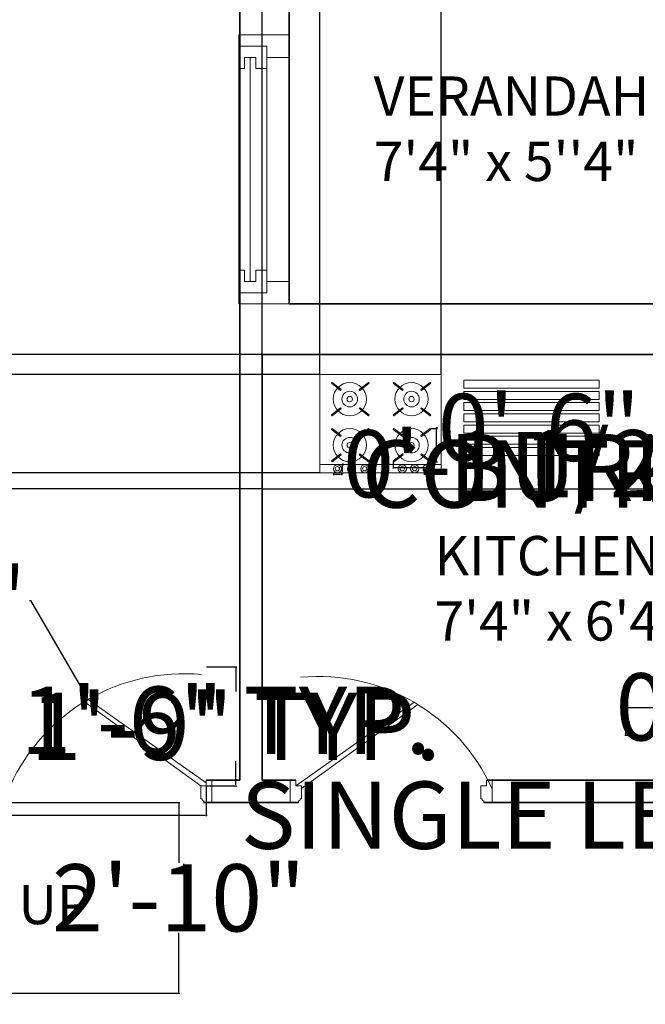
# Model space of a CAD drawing. Units: inches. Extents: x 1063 to 2718, y 423 to 1923.
# Tile 4 of 7: x 1268 to 1379, y 862 to 1038. Entities that reach past the tile are written whole.
import ezdxf

# ---------------------------------------------------------------- set-up
doc = ezdxf.new("R2010")
doc.units = ezdxf.units.IN
doc.header["$LTSCALE"] = 6
doc.header["$MEASUREMENT"] = 0
for name, color, linetype, lineweight in [('A-ANNO-DIMS', 2, 'Continuous', 18), ('A-ANNO-TEXT', 7, 'Continuous', 18), ('A-AREA-IDEN', 7, 'Continuous', 18), ('A-DOOR', 2, 'Continuous', 18), ('A-EQPM', 4, 'Continuous', 18), ('A-FLOR-CASE', 7, 'Continuous', 25), ('A-FLOR-FIXT', 4, 'Continuous', 18), ('A-GLAZ', 4, 'Continuous', 18), ('A-WALL', 7, 'Continuous', 35)]:
    doc.layers.add(name, color=color, linetype=linetype, lineweight=lineweight)
doc.styles.get("Standard").update_dxf_attribs({"font": 'arial.ttf'})
doc.dimstyles.get("Standard").update_dxf_attribs({"dimtxt": 12, "dimasz": 0.18, "dimexe": 0.18, "dimexo": 0.0625, "dimgap": 0.09, "dimtad": 0, "dimtih": 1, "dimtoh": 1, "dimdec": 1, "dimzin": 0, "dimdsep": 46, "dimlunit": 3, "dimtxsty": 'Standard', "dimcen": 0.09, "dimadec": 0, "dimazin": 0, "dimtfac": 1, "dimtdec": 1, "dimtofl": 0, "dimtmove": 0, "dimatfit": 3, "dimfxl": 1, "dimtolj": 1, "dimtzin": 0, "dimarcsym": 0})

# ---------------------------------------------------------------- blocks, each defined once
blk = doc.blocks.new('WIN-48-SLIDING')
at = {"ltscale": 6}
for p, q in [((0, 9), (4, 9)), ((4, 9), (4, 5)), ((48, 9), (44, 9)), ((44, 9), (44, 5)), ((4, 5), (2, 5)), ((2, 5), (2, 0)), ((4, 5), (44, 5)), ((4, 5), (6, 5)), ((6, 5), (6, 3)), ((44, 5), (42, 5)), ((42, 5), (42, 3)), ((44, 5), (46, 5)), ((46, 5), (46, 0)), ((6, 3), (4, 3)), ((4, 3), (4, 1)), ((4, 2), (44, 2)), ((42, 3), (44, 3)), ((44, 3), (44, 1)), ((4, 1), (6, 1)), ((6, 1), (6, 0)), ((44, 1), (42, 1)), ((42, 1), (42, 0)), ((48, 0), (0, 0)), ((2, 0), (46, 0))]:
    blk.add_line(p, q, dxfattribs=at)
blk.add_lwpolyline([(48, 0), (48, 9), (0, 9), (0, 0)], dxfattribs=at)
blk = doc.blocks.new('DOOR-JAMB-4')
at = {"ltscale": 6}
for p, q in [((0, 0), (0, 4)), ((1, 4), (1, 3)), ((1, 3), (2, 3)), ((2, 3), (2, 0.69)), ((1.46, 0), (1.46, 0.33)), ((1.46, 0.33), (1.56, 0.33)), ((1.76, 0.53), (1.76, 0.69)), ((1.76, 0.69), (2, 0.69))]:
    blk.add_line(p, q, dxfattribs=at)
blk.add_arc((1.56, 0.53), 0.2, 270, 0, dxfattribs=at)
blk = doc.blocks.new('DOOR-LEAF-SINGLE-SWING')
at = {"ltscale": 6}
for p, q in [((34, 0), (13.24, 15)), ((35, 0.5), (13.9, 15.4))]:
    blk.add_line(p, q, dxfattribs=at)
blk.add_arc((31.02, -14.03), 34.04, 84.6951, 155.6613, dxfattribs=at)
blk = doc.blocks.new('COOKTOP-BURNER')
at = {"ltscale": 6}
for points in [[(1.65, 4.53), (0, 5.8), (0.13, 5.97), (1.77, 4.69)], [(5.08, 4.53), (6.73, 5.8), (6.61, 5.97), (4.96, 4.69)], [(1.65, 1.44), (0, 0.16), (0.13, 0), (1.77, 1.28)], [(5.08, 1.44), (6.73, 0.16), (6.61, 0), (4.96, 1.28)]]:
    blk.add_lwpolyline(points, close=True, dxfattribs=at)
for radius in [2.96, 1.39, 0.48]:
    blk.add_circle((3.28, 2.98), radius, dxfattribs=at)
blk = doc.blocks.new('COOKTOP-CONTROL')
at = {"ltscale": 6}
for radius in [0.719, 0.388]:
    blk.add_circle((0.72, 0.72), radius, dxfattribs=at)
blk = doc.blocks.new('*D26')
at = {"layer": 'A-ANNO-DIMS', "color": 0, "lineweight": -2, "ltscale": 6, "transparency": 16777216}
for p, q in [((1174.93, 910.18), (1174.93, 913)), ((1175.11, 912.82), (1192.75, 912.82)), ((1192.93, 910.18), (1192.93, 913)), ((1192.93, 912.82), (1193.11, 912.82))]:
    blk.add_line(p, q, dxfattribs=at)
at = {"layer": 'A-ANNO-DIMS', "color": 0, "ltscale": 6, "transparency": 16777216}
for points in [[(1175.11, 912.85), (1175.11, 912.79), (1174.93, 912.82)], [(1192.75, 912.85), (1192.75, 912.79), (1192.93, 912.82)]]:
    blk.add_solid(points, dxfattribs=at)
at = {"layer": 'Defpoints', "color": 0, "ltscale": 6, "transparency": 16777216}
for p in [(1192.93, 912.82), (1174.93, 910.12), (1192.93, 910.12)]:
    blk.add_point(p, dxfattribs=at)
at = {"layer": 'A-ANNO-DIMS', "color": 0, "ltscale": 6, "transparency": 16777216, "insert": (1268.35, 912.82), "char_height": 12, "attachment_point": 5}
blk.add_mtext('\\A1;COLUMN 1\'-6" TYP.', dxfattribs=at)
blk = doc.blocks.new('*D34')
at = {"layer": 'A-ANNO-DIMS', "color": 0, "lineweight": -2, "ltscale": 6, "transparency": 16777216}
for p, q in [((1323.62, 956.91), (1323.62, 956.58)), ((1323.8, 956.76), (1324.88, 956.76)), ((1325.06, 956.91), (1325.06, 956.58)), ((1325.06, 956.76), (1325.24, 956.76))]:
    blk.add_line(p, q, dxfattribs=at)
at = {"layer": 'A-ANNO-DIMS', "color": 0, "ltscale": 6, "transparency": 16777216}
for points in [[(1323.8, 956.79), (1323.8, 956.73), (1323.62, 956.76)], [(1324.88, 956.79), (1324.88, 956.73), (1325.06, 956.76)]]:
    blk.add_solid(points, dxfattribs=at)
at = {"layer": 'Defpoints', "color": 0, "ltscale": 6, "transparency": 16777216}
for p in [(1323.62, 956.97), (1325.06, 956.97), (1325.06, 956.76)]:
    blk.add_point(p, dxfattribs=at)
at = {"layer": 'A-ANNO-DIMS', "color": 0, "ltscale": 6, "transparency": 16777216, "insert": (1419.12, 956.76), "char_height": 12, "attachment_point": 5}
blk.add_mtext('\\A1;CONTROL 0\'-1 1/2" TYP.', dxfattribs=at)
blk = doc.blocks.new('*D35')
at = {"layer": 'A-ANNO-DIMS', "color": 0, "lineweight": -2, "ltscale": 6, "transparency": 16777216}
for p, q in [((1325.12, 958.41), (1325.45, 958.41)), ((1325.27, 958.41), (1325.27, 958.59)), ((1325.27, 958.59), (1325.45, 958.59)), ((1325.27, 957.15), (1325.27, 958.23)), ((1325.12, 956.97), (1325.45, 956.97))]:
    blk.add_line(p, q, dxfattribs=at)
at = {"layer": 'A-ANNO-DIMS', "color": 0, "ltscale": 6, "transparency": 16777216}
for points in [[(1325.24, 958.23), (1325.3, 958.23), (1325.27, 958.41)], [(1325.24, 957.15), (1325.3, 957.15), (1325.27, 956.97)]]:
    blk.add_solid(points, dxfattribs=at)
at = {"layer": 'Defpoints', "color": 0, "ltscale": 6, "transparency": 16777216}
for p in [(1325.06, 958.41), (1325.27, 958.41), (1325.06, 956.97)]:
    blk.add_point(p, dxfattribs=at)
at = {"layer": 'A-ANNO-DIMS', "color": 0, "ltscale": 6, "transparency": 16777216, "insert": (1376.1, 958.59), "char_height": 12, "attachment_point": 5}
blk.add_mtext('\\A1;0\'-1 1/2" TYP.', dxfattribs=at)
blk = doc.blocks.new('*D36')
at = {"layer": 'A-ANNO-DIMS', "color": 0, "lineweight": -2, "ltscale": 6, "transparency": 16777216}
for p, q in [((1334.27, 958.87), (1334.27, 957.74)), ((1334.45, 957.92), (1340.83, 957.92)), ((1341.01, 958.87), (1341.01, 957.74)), ((1341.01, 957.92), (1341.19, 957.92))]:
    blk.add_line(p, q, dxfattribs=at)
at = {"layer": 'A-ANNO-DIMS', "color": 0, "ltscale": 6, "transparency": 16777216}
for points in [[(1334.45, 957.95), (1334.45, 957.89), (1334.27, 957.92)], [(1340.83, 957.95), (1340.83, 957.89), (1341.01, 957.92)]]:
    blk.add_solid(points, dxfattribs=at)
at = {"layer": 'Defpoints', "color": 0, "ltscale": 6, "transparency": 16777216}
for p in [(1334.27, 958.93), (1341.01, 958.93), (1341.01, 957.92)]:
    blk.add_point(p, dxfattribs=at)
at = {"layer": 'A-ANNO-DIMS', "color": 0, "ltscale": 6, "transparency": 16777216, "insert": (1429.29, 957.92), "char_height": 12, "attachment_point": 5}
blk.add_mtext('\\A1;BURNER 0\'-6 1/2" TYP.', dxfattribs=at)
blk = doc.blocks.new('*D37')
at = {"layer": 'A-ANNO-DIMS', "color": 0, "lineweight": -2, "ltscale": 6, "transparency": 16777216}
for p, q in [((1341.07, 964.9), (1342.2, 964.9)), ((1342.02, 964.9), (1342.02, 965.08)), ((1342.02, 965.08), (1342.2, 965.08)), ((1342.02, 959.11), (1342.02, 964.72)), ((1341.07, 958.93), (1342.2, 958.93))]:
    blk.add_line(p, q, dxfattribs=at)
at = {"layer": 'A-ANNO-DIMS', "color": 0, "ltscale": 6, "transparency": 16777216}
for points in [[(1341.99, 964.72), (1342.05, 964.72), (1342.02, 964.9)], [(1341.99, 959.11), (1342.05, 959.11), (1342.02, 958.93)]]:
    blk.add_solid(points, dxfattribs=at)
at = {"layer": 'Defpoints', "color": 0, "ltscale": 6, "transparency": 16777216}
for p in [(1341.01, 964.9), (1342.02, 964.9), (1341.01, 958.93)]:
    blk.add_point(p, dxfattribs=at)
at = {"layer": 'A-ANNO-DIMS', "color": 0, "ltscale": 6, "transparency": 16777216, "insert": (1378.86, 965.08), "char_height": 12, "attachment_point": 5}
blk.add_mtext('\\A1;0\'-6" TYP.', dxfattribs=at)
blk = doc.blocks.new('*D42')
at = {"layer": 'A-ANNO-DIMS', "color": 0, "lineweight": -2, "ltscale": 6, "transparency": 16777216}
for p, q in [((1265.93, 901.06), (1265.93, 895.69)), ((1300.93, 901.06), (1300.93, 895.69)), ((1266.11, 895.87), (1300.75, 895.87)), ((1300.93, 895.87), (1301.11, 895.87))]:
    blk.add_line(p, q, dxfattribs=at)
at = {"layer": 'A-ANNO-DIMS', "color": 0, "ltscale": 6, "transparency": 16777216}
for points in [[(1266.11, 895.9), (1266.11, 895.84), (1265.93, 895.87)], [(1300.75, 895.9), (1300.75, 895.84), (1300.93, 895.87)]]:
    blk.add_solid(points, dxfattribs=at)
at = {"layer": 'Defpoints', "color": 0, "ltscale": 6, "transparency": 16777216}
for p in [(1265.93, 901.12), (1300.93, 901.12), (1300.93, 895.87)]:
    blk.add_point(p, dxfattribs=at)
at = {"layer": 'A-ANNO-DIMS', "color": 0, "ltscale": 6, "transparency": 16777216, "insert": (1398.77, 895.87), "char_height": 12, "attachment_point": 5}
blk.add_mtext('\\A1;SINGLE LEAF 2\'-11" TYP.', dxfattribs=at)
blk = doc.blocks.new('*D43')
at = {"layer": 'A-ANNO-DIMS', "color": 0, "lineweight": -2, "ltscale": 6, "transparency": 16777216}
for p, q in [((1300.99, 922.33), (1306.36, 922.33)), ((1306.18, 922.15), (1306.18, 917.94)), ((1306.18, 901.3), (1306.18, 905.51)), ((1300.99, 901.12), (1306.36, 901.12))]:
    blk.add_line(p, q, dxfattribs=at)
at = {"layer": 'A-ANNO-DIMS', "color": 0, "ltscale": 6, "transparency": 16777216}
for points in [[(1306.15, 922.15), (1306.21, 922.15), (1306.18, 922.33)], [(1306.15, 901.3), (1306.21, 901.3), (1306.18, 901.12)]]:
    blk.add_solid(points, dxfattribs=at)
at = {"layer": 'Defpoints', "color": 0, "ltscale": 6, "transparency": 16777216}
for p in [(1300.93, 922.33), (1306.18, 922.33), (1300.93, 901.12)]:
    blk.add_point(p, dxfattribs=at)
at = {"layer": 'A-ANNO-DIMS', "color": 0, "ltscale": 6, "transparency": 16777216, "insert": (1306.18, 911.72), "char_height": 12, "attachment_point": 5}
blk.add_mtext('\\A1;1\'-9" TYP.', dxfattribs=at)
blk = doc.blocks.new('*D57')
at = {"layer": 'A-ANNO-DIMS', "color": 0, "lineweight": -2, "ltscale": 6, "transparency": 16777216}
for p, q in [((1263.99, 898.12), (1296.21, 898.12)), ((1296.03, 897.94), (1296.03, 887.34)), ((1296.03, 864.3), (1296.03, 874.9)), ((1263.99, 864.12), (1296.21, 864.12))]:
    blk.add_line(p, q, dxfattribs=at)
at = {"layer": 'A-ANNO-DIMS', "color": 0, "ltscale": 6, "transparency": 16777216}
for points in [[(1296, 897.94), (1296.06, 897.94), (1296.03, 898.12)], [(1296, 864.3), (1296.06, 864.3), (1296.03, 864.12)]]:
    blk.add_solid(points, dxfattribs=at)
at = {"layer": 'Defpoints', "color": 0, "ltscale": 6, "transparency": 16777216}
for p in [(1263.93, 898.12), (1263.93, 864.12), (1296.03, 864.12)]:
    blk.add_point(p, dxfattribs=at)
at = {"layer": 'A-ANNO-DIMS', "color": 0, "ltscale": 6, "transparency": 16777216, "insert": (1296.03, 881.12), "char_height": 12, "attachment_point": 5}
blk.add_mtext('\\A1;2\'-10"', dxfattribs=at)
blk = doc.blocks.new('*D59')
at = {"layer": 'A-ANNO-DIMS', "color": 0, "lineweight": -2, "ltscale": 6, "transparency": 16777216}
for p, q in [((1310.86, 978.12), (1118.65, 978.12)), ((1118.83, 977.94), (1118.83, 972.34)), ((1118.83, 954.3), (1118.83, 959.9)), ((1310.86, 954.12), (1118.65, 954.12))]:
    blk.add_line(p, q, dxfattribs=at)
at = {"layer": 'A-ANNO-DIMS', "color": 0, "ltscale": 6, "transparency": 16777216}
for points in [[(1118.8, 977.94), (1118.86, 977.94), (1118.83, 978.12)], [(1118.8, 954.3), (1118.86, 954.3), (1118.83, 954.12)]]:
    blk.add_solid(points, dxfattribs=at)
at = {"layer": 'Defpoints', "color": 0, "ltscale": 6, "transparency": 16777216}
for p in [(1310.93, 978.12), (1118.83, 954.12), (1310.93, 954.12)]:
    blk.add_point(p, dxfattribs=at)
at = {"layer": 'A-ANNO-DIMS', "color": 0, "ltscale": 6, "transparency": 16777216, "insert": (1118.83, 966.12), "char_height": 12, "attachment_point": 5}
blk.add_mtext('\\A1;2\'-0"', dxfattribs=at)
blk = doc.blocks.new('*D60')
at = {"layer": 'A-ANNO-DIMS', "color": 0, "lineweight": -2, "ltscale": 6, "transparency": 16777216}
for p, q in [((1321.21, 974.62), (1321.21, 1117.4)), ((1321.39, 1117.22), (1342.7, 1117.22)), ((1342.88, 974.62), (1342.88, 1117.4)), ((1342.88, 1117.22), (1343.06, 1117.22))]:
    blk.add_line(p, q, dxfattribs=at)
at = {"layer": 'A-ANNO-DIMS', "color": 0, "ltscale": 6, "transparency": 16777216}
for points in [[(1321.39, 1117.25), (1321.39, 1117.19), (1321.21, 1117.22)], [(1342.7, 1117.25), (1342.7, 1117.19), (1342.88, 1117.22)]]:
    blk.add_solid(points, dxfattribs=at)
at = {"layer": 'Defpoints', "color": 0, "ltscale": 6, "transparency": 16777216}
for p in [(1342.88, 1117.22), (1321.21, 974.55), (1342.88, 974.55)]:
    blk.add_point(p, dxfattribs=at)
at = {"layer": 'A-ANNO-DIMS', "color": 0, "ltscale": 6, "transparency": 16777216, "insert": (1372.52, 1117.22), "char_height": 12, "attachment_point": 5}
blk.add_mtext('\\A1;1\'-9 1/2"', dxfattribs=at)
blk = doc.blocks.new('*D61')
at = {"layer": 'A-ANNO-DIMS', "color": 0, "lineweight": -2, "ltscale": 6, "transparency": 16777216}
for p, q in [((1321.15, 974.55), (1118.65, 974.55)), ((1118.83, 974.37), (1118.83, 972.07)), ((1118.83, 957.17), (1118.83, 959.48)), ((1321.15, 956.99), (1118.65, 956.99))]:
    blk.add_line(p, q, dxfattribs=at)
at = {"layer": 'A-ANNO-DIMS', "color": 0, "ltscale": 6, "transparency": 16777216}
for points in [[(1118.8, 974.37), (1118.86, 974.37), (1118.83, 974.55)], [(1118.8, 957.17), (1118.86, 957.17), (1118.83, 956.99)]]:
    blk.add_solid(points, dxfattribs=at)
at = {"layer": 'Defpoints', "color": 0, "ltscale": 6, "transparency": 16777216}
for p in [(1118.83, 974.55), (1321.21, 974.55), (1321.21, 956.99)]:
    blk.add_point(p, dxfattribs=at)
at = {"layer": 'A-ANNO-DIMS', "color": 0, "ltscale": 6, "transparency": 16777216, "insert": (1118.83, 965.77), "char_height": 12, "attachment_point": 5}
blk.add_mtext('\\A1;1\'-5 1/2"', dxfattribs=at)
blk = doc.blocks.new('*D64')
at = {"layer": 'A-ANNO-DIMS', "color": 0, "lineweight": -2, "ltscale": 6, "transparency": 16777216}
for p, q in [((1310.93, 978.18), (1310.93, 1117.4)), ((1311.11, 1117.22), (1321.03, 1117.22)), ((1321.21, 974.62), (1321.21, 1117.4)), ((1321.21, 1117.22), (1321.39, 1117.22))]:
    blk.add_line(p, q, dxfattribs=at)
at = {"layer": 'A-ANNO-DIMS', "color": 0, "ltscale": 6, "transparency": 16777216}
for points in [[(1311.11, 1117.25), (1311.11, 1117.19), (1310.93, 1117.22)], [(1321.03, 1117.25), (1321.03, 1117.19), (1321.21, 1117.22)]]:
    blk.add_solid(points, dxfattribs=at)
at = {"layer": 'Defpoints', "color": 0, "ltscale": 6, "transparency": 16777216}
for p in [(1321.21, 1117.22), (1310.93, 978.12), (1321.21, 974.55)]:
    blk.add_point(p, dxfattribs=at)
at = {"layer": 'A-ANNO-DIMS', "color": 0, "ltscale": 6, "transparency": 16777216, "insert": (1356.07, 1117.22), "char_height": 12, "attachment_point": 5}
blk.add_mtext('\\A1;0\'-10 1/2"', dxfattribs=at)
blk = doc.blocks.new('*D72')
at = {"layer": 'A-ANNO-DIMS', "color": 0, "lineweight": -2, "ltscale": 6, "transparency": 16777216}
for p, q in [((1407.86, 915.02), (1375.65, 915.02)), ((1375.83, 915.02), (1375.83, 915.2)), ((1375.83, 915.2), (1376.01, 915.2)), ((1375.83, 910.3), (1375.83, 914.84)), ((1407.86, 910.12), (1375.65, 910.12))]:
    blk.add_line(p, q, dxfattribs=at)
at = {"layer": 'A-ANNO-DIMS', "color": 0, "ltscale": 6, "transparency": 16777216}
for points in [[(1375.8, 914.84), (1375.86, 914.84), (1375.83, 915.02)], [(1375.8, 910.3), (1375.86, 910.3), (1375.83, 910.12)]]:
    blk.add_solid(points, dxfattribs=at)
at = {"layer": 'Defpoints', "color": 0, "ltscale": 6, "transparency": 16777216}
for p in [(1375.83, 915.02), (1407.93, 915.02), (1407.93, 910.12)]:
    blk.add_point(p, dxfattribs=at)
at = {"layer": 'A-ANNO-DIMS', "color": 0, "ltscale": 6, "transparency": 16777216, "insert": (1392.05, 915.2), "char_height": 12, "attachment_point": 5}
blk.add_mtext('\\A1;0\'-5"', dxfattribs=at)
blk = doc.blocks.new('*D73')
at = {"layer": 'A-ANNO-DIMS', "color": 0, "lineweight": -2, "ltscale": 6, "transparency": 16777216}
for p, q in [((1269.38, 934.18), (1269.56, 934.18)), ((1269.56, 934.18), (1279.74, 916.67)), ((1296.85, 887.09), (1297.03, 887.09)), ((1296.94, 887), (1296.94, 887.18))]:
    blk.add_line(p, q, dxfattribs=at)
at = {"layer": 'A-ANNO-DIMS', "color": 0, "ltscale": 6, "transparency": 16777216}
blk.add_solid([(1279.77, 916.69), (1279.71, 916.66), (1279.83, 916.52)], dxfattribs=at)
at = {"layer": 'Defpoints', "color": 0, "ltscale": 6, "transparency": 16777216}
for p in [(1279.83, 916.52), (1296.94, 887.09)]:
    blk.add_point(p, dxfattribs=at)
at = {"layer": 'A-ANNO-DIMS', "color": 0, "ltscale": 6, "transparency": 16777216, "insert": (1229.94, 934.18), "char_height": 12, "attachment_point": 5}
blk.add_mtext('\\A1;2X R2\'-10"', dxfattribs=at)

msp = doc.modelspace()

# ---------------------------------------------------------------- linework, layer by layer
at = {"layer": 'A-EQPM', "ltscale": 6}
msp.add_line((1321.21, 958.44), (1342.88, 958.44), dxfattribs=at)
msp.add_lwpolyline([(1321.21, 974.55), (1342.88, 974.55), (1342.88, 956.99), (1321.21, 956.99)], close=True, dxfattribs=at)
at = {"layer": 'A-FLOR-CASE'}
msp.add_line((1310.93, 954.12), (1398.93, 954.12), dxfattribs=at)
at = {"layer": 'A-FLOR-FIXT', "ltscale": 6}
for points in [[(1346.87, 973.51), (1371.07, 973.51), (1371.07, 972.08), (1346.87, 972.08)], [(1346.87, 971.51), (1371.07, 971.51), (1371.07, 970.08), (1346.87, 970.08)], [(1346.87, 969.51), (1371.07, 969.51), (1371.07, 968.08), (1346.87, 968.08)], [(1346.87, 967.51), (1371.07, 967.51), (1371.07, 966.08), (1346.87, 966.08)], [(1346.87, 965.51), (1371.07, 965.51), (1371.07, 964.08), (1346.87, 964.08)], [(1346.87, 963.51), (1371.07, 963.51), (1371.07, 962.08), (1346.87, 962.08)], [(1346.87, 961.51), (1371.07, 961.51), (1371.07, 960.08), (1346.87, 960.08)]]:
    msp.add_lwpolyline(points, close=True, dxfattribs=at)
at = {"layer": 'A-WALL'}
for p, q in [((1315.75, 1055.12), (1315.75, 987.12)), ((1306.93, 1046.12), (1306.93, 902.12)), ((1315.75, 987.12), (1407.93, 987.12)), ((1310.93, 978.12), (1310.93, 902.12)), ((1310.93, 978.12), (1398.93, 978.12)), ((1310.93, 902.12), (1316.93, 902.12))]:
    msp.add_line(p, q, dxfattribs=at)
at = {"layer": 'A-WALL', "ltscale": 6}
for p, q in [((1306.93, 902.12), (1300.93, 902.12)), ((1389.93, 902.12), (1350.93, 902.12)), ((1300.46, 898.12), (1317.39, 898.12)), ((1350.46, 898.12), (1398.93, 898.12))]:
    msp.add_line(p, q, dxfattribs=at)

# ---------------------------------------------------------------- block references
at = {"layer": 'A-DOOR'}
for name, p in [('DOOR-LEAF-SINGLE-SWING', (1265.93, 901.12)), ('DOOR-JAMB-4', (1315.93, 898.12))]:
    msp.add_blockref(name, p, dxfattribs=at)
at = {"layer": 'A-DOOR', "extrusion": (0, 0, -1), "zscale": -1}
for name, p in [('DOOR-LEAF-SINGLE-SWING', (-1351.93, 900.62)), ('DOOR-JAMB-4', (-1301.93, 898.12)), ('DOOR-JAMB-4', (-1351.93, 898.12))]:
    msp.add_blockref(name, p, dxfattribs=at)
at = {"layer": 'A-EQPM'}
for name, p in [('COOKTOP-BURNER', (1323.26, 967.15)), ('COOKTOP-BURNER', (1334.28, 967.15)), ('COOKTOP-BURNER', (1323.26, 958.93)), ('COOKTOP-BURNER', (1334.28, 958.93)), ('COOKTOP-CONTROL', (1323.62, 956.98)), ('COOKTOP-CONTROL', (1326.11, 956.98)), ('COOKTOP-CONTROL', (1328.5, 956.98)), ('COOKTOP-CONTROL', (1335.2, 956.98)), ('COOKTOP-CONTROL', (1337.4, 956.98)), ('COOKTOP-CONTROL', (1339.61, 956.98))]:
    msp.add_blockref(name, p, dxfattribs=at)
at = {"layer": 'A-GLAZ', "rotation": 270.0000000000011}
msp.add_blockref('WIN-48-SLIDING', (1306.75, 1035.12), dxfattribs=at)

# ---------------------------------------------------------------- texts
at = {"layer": 'A-ANNO-TEXT', "ltscale": 6, "insert": (1267.39, 883.42), "char_height": 7, "attachment_point": 1}
msp.add_mtext_dynamic_manual_height_columns('UP', width=175.2385, gutter_width=1, heights=[0], dxfattribs=at)
at = {"layer": 'A-AREA-IDEN', "ltscale": 6, "char_height": 7, "attachment_point": 1}
for s, insert in [('VERANDAH\\P7\'4" x 5\'\'4"', (1330.81, 1027.72)), ('KITCHEN\\P7\'4" x 6\'4"', (1341.66, 945.7))]:
    msp.add_mtext_dynamic_manual_height_columns(s, width=175.2385, gutter_width=1, heights=[0], dxfattribs=dict(at, insert=insert))

# ---------------------------------------------------------------- dimensions: what is measured, and where the dimension line sits
at = {"layer": 'A-ANNO-DIMS', "ltscale": 6}
for base, p1, p2, picture, middle in [((1321.21, 1117.22), (1310.93, 978.12), (1321.21, 974.55), '*D64', (1356.07, 1117.22)), ((1342.88, 1117.22), (1321.21, 974.55), (1342.88, 974.55), '*D60', (1372.52, 1117.22))]:
    dim = msp.add_linear_dim(base=base, p1=p1, p2=p2, dimstyle='Standard', override={"dimdec": 1, "dimlfac": 1, "dimrnd": 0, "dimzin": 1, "dimdsep": 46, "dimlunit": 4, "dimfrac": 2}, dxfattribs=at)
    dim.commit()
    dim.dimension.update_dxf_attribs({"geometry": picture, "text_midpoint": middle})
for base, p1, p2, text, picture, middle in [((1325.06, 956.76), (1323.62, 956.97), (1325.06, 956.97), 'CONTROL <> TYP.', '*D34', (1419.12, 956.76)), ((1341.01, 957.92), (1334.27, 958.93), (1341.01, 958.93), 'BURNER <> TYP.', '*D36', (1429.29, 957.92)), ((1192.93, 912.82), (1174.93, 910.12), (1192.93, 910.12), 'COLUMN <> TYP.', '*D26', (1268.35, 912.82)), ((1300.93, 895.87), (1265.93, 901.12), (1300.93, 901.12), 'SINGLE LEAF <> TYP.', '*D42', (1398.77, 895.87))]:
    dim = msp.add_linear_dim(base=base, p1=p1, p2=p2, text=text, dimstyle='Standard', override={"dimdec": 1, "dimlfac": 1, "dimrnd": 0, "dimzin": 1, "dimdsep": 46, "dimlunit": 4, "dimfrac": 2}, dxfattribs=at)
    dim.commit()
    dim.dimension.update_dxf_attribs({"geometry": picture, "text_midpoint": middle})
for base, p1, p2, picture, middle in [((1325.27, 958.41), (1325.06, 956.97), (1325.06, 958.41), '*D35', (1376.1, 958.59)), ((1342.02, 964.9), (1341.01, 958.93), (1341.01, 964.9), '*D37', (1378.86, 965.08)), ((1306.18, 922.33), (1300.93, 901.12), (1300.93, 922.33), '*D43', (1306.18, 911.72))]:
    dim = msp.add_linear_dim(base=base, p1=p1, p2=p2, angle=90, text='<> TYP.', dimstyle='Standard', override={"dimdec": 1, "dimlfac": 1, "dimrnd": 0, "dimzin": 1, "dimdsep": 46, "dimlunit": 4, "dimfrac": 2}, dxfattribs=at)
    dim.commit()
    dim.dimension.update_dxf_attribs({"geometry": picture, "text_midpoint": middle})
for base, p1, p2, angle, picture, middle in [((1118.83, 974.55), (1321.21, 956.99), (1321.21, 974.55), 90, '*D61', (1118.83, 965.77)), ((1118.83, 954.12), (1310.93, 978.12), (1310.93, 954.12), 90, '*D59', (1118.83, 966.12)), ((1375.83, 915.02), (1407.93, 910.12), (1407.93, 915.02), 90, '*D72', (1392.05, 915.2)), ((1296.03, 864.12), (1263.93, 898.12), (1263.93, 864.12), 270, '*D57', (1296.03, 881.12))]:
    dim = msp.add_linear_dim(base=base, p1=p1, p2=p2, angle=angle, dimstyle='Standard', override={"dimdec": 1, "dimlfac": 1, "dimrnd": 0, "dimzin": 1, "dimdsep": 46, "dimlunit": 4, "dimfrac": 2}, dxfattribs=at)
    dim.commit()
    dim.dimension.update_dxf_attribs({"geometry": picture, "text_midpoint": middle})
dim = msp.add_radius_dim(center=(1296.94, 887.09), mpoint=(1279.83, 916.52), text='2X <>', dimstyle='Standard', override={"dimdec": 1, "dimlfac": 1, "dimrnd": 0, "dimzin": 1, "dimdsep": 46, "dimlunit": 4, "dimfrac": 2}, dxfattribs=at)
dim.commit()
dim.dimension.update_dxf_attribs({"geometry": '*D73', "text_midpoint": (1229.94, 934.18), "dimtype": 164})

doc.saveas('drawing.dxf')
